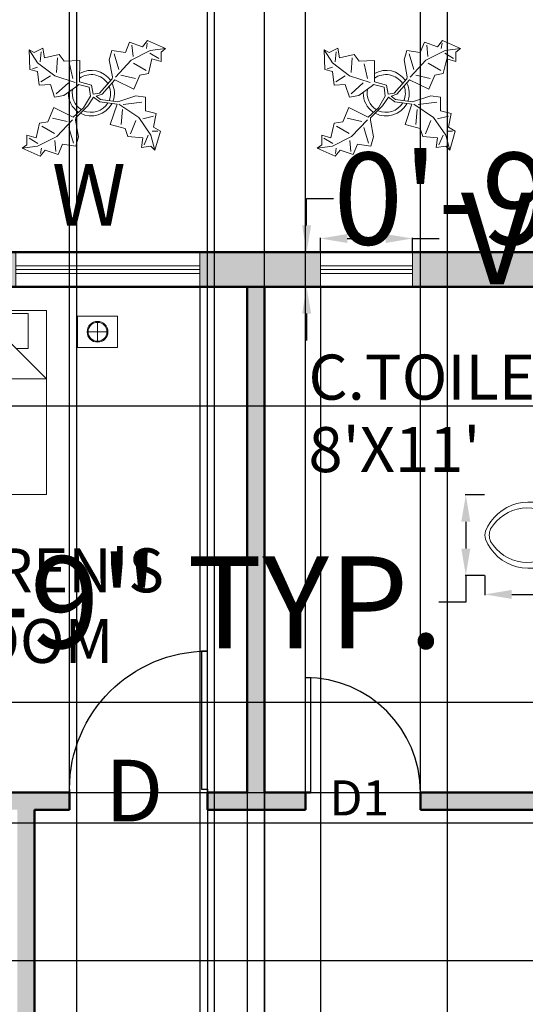
# Model space of a CAD drawing. Units: inches. Extents: x -166 to 1001, y 0 to 688.
# Tile 5 of 11: x 97 to 229, y 287 to 544. Entities that reach past the tile are written whole.
import ezdxf

# ---------------------------------------------------------------- set-up
doc = ezdxf.new("R2010")
doc.units = ezdxf.units.IN
doc.header["$MEASUREMENT"] = 0
for name, color, linetype, lineweight in [('A-ANNO-DIMS', 1, 'Continuous', 18), ('A-ANNO-TEXT', 2, 'Continuous', 25), ('A-AREA-IDEN', 2, 'Continuous', 25), ('A-DOOR', 6, 'Continuous', 25), ('A-FLOR-FIXT', 11, 'Continuous', 18), ('A-GLAZ', 130, 'Continuous', 18), ('A-GLAZ-VENT', 130, 'Continuous', 18), ('A-WALL-PATT', 5, 'Continuous', 13), ('FURNITURE', 11, 'Continuous', 18), ('TREES', 80, 'Continuous', 13), ('WALLS', 250, 'Continuous', 50)]:
    doc.layers.add(name, color=color, linetype=linetype, lineweight=lineweight)
doc.styles.get("Standard").update_dxf_attribs({"font": 'arial.ttf'})
doc.dimstyles.get("Standard").update_dxf_attribs({"dimtxt": 24, "dimasz": 7, "dimexe": 0.18, "dimexo": 0.0625, "dimgap": 0.09, "dimtad": 0, "dimtih": 1, "dimtoh": 1, "dimdec": 0, "dimzin": 0, "dimdsep": 46, "dimlunit": 3, "dimtxsty": 'Standard', "dimcen": 0.09, "dimadec": 0, "dimazin": 0, "dimtfac": 1, "dimtdec": 0, "dimtofl": 0, "dimtmove": 0, "dimatfit": 3, "dimfxl": 1, "dimtolj": 1, "dimtzin": 0, "dimarcsym": 0})

# ---------------------------------------------------------------- blocks, each defined once
blk = doc.blocks.new('*U6')
for p, q in [((0, 0), (0, -6)), ((40, 0), (40, -6))]:
    blk.add_line(p, q)
blk.add_lwpolyline([(0, 0), (0, 40), (1.75, 40), (1.75, 0)], close=True)
blk.add_arc((0, 0), 40, 0, 90)
blk = doc.blocks.new('Bed - Queen')
for p, q in [((0, -80.00003), (0, 0)), ((0, 0), (59.99999, 0)), ((59.99999, 0), (59.99999, -80.00003)), ((7.99999, -1.2), (28.79998, -1.2)), ((7.99999, -14.4), (7.99999, -1.2)), ((28.79998, -1.2), (28.79998, -14.4)), ((31.19999, -1.2), (51.99999, -1.2)), ((31.19999, -14.4), (31.19999, -1.2)), ((51.99999, -1.2), (51.99999, -16.4)), ((0, -14.4), (44.8, -14.4)), ((44.8, -16.8), (0, -16.8)), ((59.99999, -29.6), (44.8, -14.4)), ((44.8, -14.4), (44.8, -29.6)), ((51.99999, -16.4), (46.79936, -16.4)), ((44.8, -29.6), (59.99999, -29.6)), ((59.99999, -80.00003), (0, -80.00003))]:
    blk.add_line(p, q)
blk = doc.blocks.new('Toilet - top')
for p, q in [((9.5, -6), (9.5, -2)), ((-10, -8.5), (-8, -8.5)), ((-10, -9.5), (-10, -8.5)), ((-7, -9.5), (-10, -9.5)), ((-8, -8.5), (-8, -8)), ((-7, -8), (-7, -9.5)), ((-4, -8), (-6, -14)), ((4, -8), (6, -14)), ((4, -14), (-4, -14))]:
    blk.add_line(p, q)
blk.add_lwpolyline([(10.5, -8), (10.5, 0), (-10.5, 0), (-10.5, -8)], close=True)
for points in [[(-9.5, -2), (-9.5, -6)], [(8.5, -1), (-8.5, -1)], [(-8.5, -7), (8.5, -7)]]:
    blk.add_lwpolyline(points)
for centre, radius, start, end in [((-8.62, -1.88), 0.884, 81.8699, 188.1301), ((8.62, -1.88), 0.884, 351.8699, 98.1301), ((-8.62, -6.12), 0.884, 171.8699, 278.1301), ((8.62, -6.12), 0.884, 261.8699, 8.1301), ((3.52, -21.58), 12.17, 141.4691, 247.9714), ((4.2, -21.82), 11.33, 136.3677, 238.9468), ((-3.52, -21.58), 12.17, 292.0284, 38.5307), ((-4.2, -21.82), 11.33, 301.053, 43.6321), ((0, -27.88), 4, 245.7318, 294.2682), ((0, -29), 4, 254.8605, 285.1395)]:
    blk.add_arc(centre, radius, start, end)
blk = doc.blocks.new('Plant - Rubber or Philodendron')
for p, q in [((8.8871, 10.7908), (9.9809, 13.4933)), ((9.9809, 13.4933), (13.3837, 12.301)), ((13.3837, 12.301), (14.68, 13.9039)), ((14.5816, 13.2037), (14.3848, 11.8033)), ((14.68, 13.9039), (19.3848, 11.8146)), ((-16.2005, 11.4774), (-13.9899, 8.1064)), ((-16.2005, 11.4774), (-14.8639, 10.7964)), ((-16.0159, 6.3329), (-16.2005, 11.4774)), ((-14.8639, 10.7964), (-12.6195, 11.8975)), ((-13.3174, 8.325), (-13.0735, 11.0065)), ((-12.6195, 11.8975), (-12.1909, 9.4345)), ((-12.1909, 9.4345), (-8.3829, 10.3)), ((-8.3829, 10.3), (-7.0549, 8.501)), ((4.6914, 8.8812), (5.3859, 11.2828)), ((5.3859, 11.2828), (8.8871, 10.7908)), ((5.9878, 10.4842), (7.1971, 6.3869)), ((15.3859, 11.3055), (10.3916, 8.7942)), ((10.5828, 12.6946), (10.8893, 9.7953)), ((15.2875, 10.6053), (17.5907, 9.2105)), ((19.3848, 11.8146), (15.3859, 11.3055)), ((19.3848, 11.8146), (18.1868, 10.9119)), ((18.1868, 10.9119), (18.1925, 8.4119)), ((-13.9899, 8.1064), (-9.5434, 4.7185)), ((-8.8369, 9.409), (-9.0894, 5.6095)), ((-7.0549, 8.501), (-3.0284, 8.6941)), ((-4.8529, 4.012), (-5.7184, 7.82)), ((-3.0284, 8.6941), (-3.0709, 3.1041)), ((4.6914, 8.8812), (5.5014, 4.4831)), ((10.3916, 8.7942), (6.2847, 4.4028)), ((14.2977, 6.1031), (10.9934, 7.9956)), ((15.7909, 9.1065), (14.8995, 5.3044)), ((18.1925, 8.4119), (15.7909, 9.1065)), ((-14.0069, 5.8704), (-16.0159, 6.3329)), ((-15.3434, 6.5514), (-13.9984, 6.9884)), ((-13.5868, 2.2894), (-14.0069, 5.8704)), ((14.8995, 5.3044), (12.7005, 4.8994)), ((-13.1329, 3.1804), (-10.6614, 4.727)), ((-9.5434, 4.7185), (-4.1917, 2.9888)), ((-9.1318, 0.0195), (-5.9793, 2.9025)), ((-3.0709, 3.1041), (0.0797, 2.3163)), ((2.1141, 0.2298), (5.4346, 3.9146)), ((6.1032, 3.6844), (2.8262, -0.031)), ((5.4346, 3.9146), (5.5014, 4.4831)), ((11.1089, 1.1958), (6.1032, 3.6844)), ((7.7005, 4.8881), (11.5025, 3.9967)), ((12.7005, 4.8994), (11.1089, 1.1958)), ((-10.6784, 2.491), (-13.5868, 2.2894)), ((-9.5858, -0.8715), (-10.6784, 2.491)), ((-7.1228, -0.443), (-3.5248, 2.2131)), ((-3.5248, 2.2131), (-3.3011, 2.4355)), ((-3.3011, 2.4355), (-0.5306, 1.7947)), ((-0.5306, 1.7947), (-0.2255, -0.5527)), ((-0.5306, 1.7947), (-0.5306, 1.7947)), ((0.0797, 2.3163), (0.4866, -0.031)), ((0.4866, -0.031), (2.1141, 0.2298)), ((-7.1228, -0.443), (-9.5858, -0.8715)), ((-2.019, -3.6148), (-0.2255, -0.5527)), ((-0.9375, -3.1608), (0.5883, -0.8135)), ((0.5883, -0.8135), (2.2447, -2.0916)), ((2.8262, -0.031), (1.3003, -0.5527)), ((1.3003, -0.5527), (2.4193, -1.4655)), ((2.2447, -2.0916), (6.7108, -2.6626)), ((2.4193, -1.4655), (6.895, -2.1175)), ((11.6605, -0.5413), (6.895, -2.1175)), ((8.3544, -2.7453), (13.1973, -2.1704)), ((11.6605, -0.5413), (14.1354, -0.8948)), ((14.1354, -0.8948), (14.1354, -4.4304)), ((-11.3237, -7.2629), (-9.7321, -3.5593)), ((-9.7321, -3.5593), (-4.7264, -6.0479)), ((-2.019, -3.6148), (-4.7264, -6.0479)), ((-4.0579, -6.2781), (-0.9375, -3.1608)), ((4.943, -7.9659), (6.7108, -2.6626)), ((12.3677, -6.1981), (7.219, -2.6772)), ((8.125, -4.0768), (7.7715, -7.9659)), ((14.1354, -4.4304), (16.9638, -5.1375)), ((16.9638, -5.1375), (16.2567, -8.673)), ((-14.4141, -11.4699), (-13.5228, -7.6679)), ((-13.5228, -7.6679), (-11.3237, -7.2629)), ((-6.3237, -7.2516), (-10.1257, -6.3602)), ((-9.0148, -11.1577), (-4.9047, -6.8122)), ((-4.1246, -6.8466), (-4.0579, -6.2781)), ((-3.3146, -11.2447), (-4.1246, -6.8466)), ((10.2463, -10.4408), (11.6605, -6.9053)), ((15.5496, -10.7943), (12.3677, -6.1981)), ((16.2567, -5.8446), (13.4283, -6.5517)), ((-12.921, -8.4665), (-9.6166, -10.359)), ((-4.611, -12.8477), (-5.8203, -8.7504)), ((8.8321, -9.0266), (4.943, -7.9659)), ((9.5392, -11.1479), (8.8321, -9.0266)), ((17.3174, -9.7337), (15.9032, -9.7337)), ((16.2567, -8.673), (18.0245, -9.7337)), ((18.0245, -9.7337), (16.6103, -14.6834)), ((-16.8157, -10.7754), (-14.4141, -11.4699)), ((-16.8101, -13.2754), (-16.8157, -10.7754)), ((-13.9107, -12.9688), (-16.2139, -11.574)), ((-14.0091, -13.669), (-9.0148, -11.1577)), ((-9.206, -15.0581), (-9.5126, -12.1588)), ((-3.3146, -11.2447), (-4.0092, -13.6463)), ((13.4283, -11.5015), (9.5392, -11.1479)), ((13.0748, -13.9763), (13.4283, -11.5015)), ((14.8425, -10.7943), (13.7819, -13.2692)), ((16.6103, -14.6834), (15.5496, -10.7943)), ((-18.008, -14.1781), (-16.8101, -13.2754)), ((-18.008, -14.1781), (-14.0091, -13.669)), ((-13.3032, -16.2674), (-18.008, -14.1781)), ((-12.0069, -14.6645), (-13.3032, -16.2674)), ((-13.2048, -15.5672), (-13.008, -14.1668)), ((-8.6042, -15.8568), (-12.0069, -14.6645)), ((-7.5103, -13.1543), (-8.6042, -15.8568)), ((-4.0092, -13.6463), (-7.5103, -13.1543)), ((15.5496, -13.6228), (13.0748, -13.9763)), ((16.6103, -14.6834), (15.5496, -13.6228))]:
    blk.add_line(p, q)
for centre, radius, start, end in [((0, 0), 6.1275, 34.37569, 120.1028), ((-0.0601, -0.2075), 5.2461, 33.82192, 124.9414), ((-0.098, 0.1364), 6.1288, 341.2017, 26.09184), ((0.0308, 0.1664), 6, 178.6147, 235.1169), ((0.0308, 0.1664), 5, 168.1647, 238.6725), ((-0.2664, 0.1682), 5.2775, 338.4094, 20.03007), ((-0.1102, 0.4886), 5.2883, 247.3711, 327.472), ((-0.0234, 0.3825), 6.1492, 242.5812, 331.2714)]:
    blk.add_arc(centre, radius, start, end)
blk = doc.blocks.new('WIN-48IN')
for p, q in [((0, 4.5), (0, 9)), ((0, 9), (0, 0)), ((48, 9), (48, 0)), ((0, 5.5), (48, 5.5)), ((0, 4.5), (48, 4.5)), ((0, 3.5), (48, 3.5))]:
    blk.add_line(p, q)
blk = doc.blocks.new('VENT-24IN')
for p, q in [((0, 4.5), (0, 9)), ((0, 9), (0, 0)), ((24, 9), (24, 0)), ((0, 5.5), (24, 5.5)), ((0, 4.5), (24, 4.5)), ((0, 3.5), (24, 3.5))]:
    blk.add_line(p, q)
blk = doc.blocks.new('BEDSIDE-TABLE-LAMP')
for p, q in [((5.2, 1.64), (5.2, 6.55)), ((2.75, 4.1), (7.66, 4.1))]:
    blk.add_line(p, q)
blk.add_lwpolyline([(0, 8.19), (10.4, 8.19), (10.4, 0), (0, 0)], close=True)
for radius in [2.71, 2.71, 2.71, 2.46]:
    blk.add_circle((5.2, 4.1), radius)
blk = doc.blocks.new('*D19')
at = {"layer": 'A-ANNO-DIMS', "color": 0, "lineweight": -2, "transparency": 16777216}
for p, q in [((175.47, 483.8), (175.47, 487.52)), ((182.47, 487.34), (192.47, 487.34)), ((199.47, 483.8), (199.47, 487.52)), ((199.47, 487.34), (206.47, 487.34))]:
    blk.add_line(p, q, dxfattribs=at)
at = {"layer": 'A-ANNO-DIMS', "color": 0, "transparency": 16777216}
for points in [[(182.47, 488.51), (182.47, 486.17), (175.47, 487.34)], [(192.47, 488.51), (192.47, 486.17), (199.47, 487.34)]]:
    blk.add_solid(points, dxfattribs=at)
at = {"layer": 'Defpoints', "color": 0, "transparency": 16777216}
for p in [(199.47, 487.34), (175.47, 483.74), (199.47, 483.74)]:
    blk.add_point(p, dxfattribs=at)
at = {"layer": 'A-ANNO-DIMS', "color": 0, "transparency": 16777216, "insert": (329.7, 487.34), "char_height": 24, "attachment_point": 5}
blk.add_mtext('\\A1;VENT 2\'-0" TYP.', dxfattribs=at)
blk = doc.blocks.new('*D20')
at = {"layer": 'A-ANNO-DIMS', "color": 0, "lineweight": -2, "transparency": 16777216}
for p, q in [((171.87, 490.74), (171.87, 497.74)), ((171.87, 497.74), (178.87, 497.74)), ((175.41, 483.74), (171.69, 483.74)), ((175.41, 474.74), (171.69, 474.74)), ((171.87, 467.74), (171.87, 460.74))]:
    blk.add_line(p, q, dxfattribs=at)
at = {"layer": 'A-ANNO-DIMS', "color": 0, "transparency": 16777216}
for points in [[(170.71, 490.74), (173.04, 490.74), (171.87, 483.74)], [(170.71, 467.74), (173.04, 467.74), (171.87, 474.74)]]:
    blk.add_solid(points, dxfattribs=at)
at = {"layer": 'Defpoints', "color": 0, "transparency": 16777216}
for p in [(171.87, 483.74), (175.47, 483.74), (175.47, 474.74)]:
    blk.add_point(p, dxfattribs=at)
at = {"layer": 'A-ANNO-DIMS', "color": 0, "transparency": 16777216, "insert": (252.11, 497.74), "char_height": 24, "attachment_point": 5}
blk.add_mtext('\\A1;0\'-9" TYP.', dxfattribs=at)
blk = doc.blocks.new('*D25')
at = {"layer": 'A-ANNO-DIMS', "color": 0, "lineweight": -2, "transparency": 16777216}
for p, q in [((218.36, 399.34), (218.36, 394.26)), ((251.4, 399.34), (251.4, 394.26)), ((225.36, 394.44), (244.4, 394.44)), ((251.4, 394.44), (258.4, 394.44))]:
    blk.add_line(p, q, dxfattribs=at)
at = {"layer": 'A-ANNO-DIMS', "color": 0, "transparency": 16777216}
for points in [[(225.36, 395.61), (225.36, 393.27), (218.36, 394.44)], [(244.4, 395.61), (244.4, 393.27), (251.4, 394.44)]]:
    blk.add_solid(points, dxfattribs=at)
at = {"layer": 'Defpoints', "color": 0, "transparency": 16777216}
for p in [(218.36, 399.4), (251.4, 399.4), (251.4, 394.44)]:
    blk.add_point(p, dxfattribs=at)
at = {"layer": 'A-ANNO-DIMS', "color": 0, "transparency": 16777216, "insert": (364.72, 394.44), "char_height": 24, "attachment_point": 5}
blk.add_mtext('\\A1;WC 2\'-9" TYP.', dxfattribs=at)
blk = doc.blocks.new('*D26')
at = {"layer": 'A-ANNO-DIMS', "color": 0, "lineweight": -2, "transparency": 16777216}
for p, q in [((218.29, 420.4), (213.22, 420.4)), ((213.4, 413.4), (213.4, 406.4)), ((218.29, 399.4), (213.22, 399.4)), ((213.4, 399.4), (213.4, 392.4)), ((213.4, 392.4), (206.4, 392.4))]:
    blk.add_line(p, q, dxfattribs=at)
at = {"layer": 'A-ANNO-DIMS', "color": 0, "transparency": 16777216}
for points in [[(212.23, 413.4), (214.57, 413.4), (213.4, 420.4)], [(212.23, 406.4), (214.57, 406.4), (213.4, 399.4)]]:
    blk.add_solid(points, dxfattribs=at)
at = {"layer": 'Defpoints', "color": 0, "transparency": 16777216}
for p in [(218.36, 420.4), (213.4, 399.4), (218.36, 399.4)]:
    blk.add_point(p, dxfattribs=at)
at = {"layer": 'A-ANNO-DIMS', "color": 0, "transparency": 16777216, "insert": (134.29, 392.4), "char_height": 24, "attachment_point": 5}
blk.add_mtext('\\A1;1\'-9" TYP.', dxfattribs=at)
blk = doc.blocks.new('*D35')
at = {"layer": 'A-ANNO-DIMS', "color": 0, "lineweight": -2, "transparency": 16777216}
for p, q in [((15.38, 483.8), (15.38, 593.07)), ((22.38, 592.89), (207.38, 592.89)), ((531.88, 592.89), (346.89, 592.89)), ((538.88, 483.8), (538.88, 593.07))]:
    blk.add_line(p, q, dxfattribs=at)
at = {"layer": 'A-ANNO-DIMS', "color": 0, "transparency": 16777216}
for points in [[(22.38, 594.06), (22.38, 591.72), (15.38, 592.89)], [(531.88, 594.06), (531.88, 591.72), (538.88, 592.89)]]:
    blk.add_solid(points, dxfattribs=at)
at = {"layer": 'Defpoints', "color": 0, "transparency": 16777216}
for p in [(538.88, 592.89), (15.38, 483.74), (538.88, 483.74)]:
    blk.add_point(p, dxfattribs=at)
at = {"layer": 'A-ANNO-DIMS', "color": 0, "transparency": 16777216, "insert": (277.13, 592.89), "char_height": 24, "attachment_point": 5}
blk.add_mtext('\\A1;43\'-7 1/2"', dxfattribs=at)
blk = doc.blocks.new('*D43')
at = {"layer": 'A-ANNO-DIMS', "color": 0, "lineweight": -2, "transparency": 16777216}
for p, q in [((160.88, 257.49), (160.88, 593.07)), ((167.88, 592.89), (201.62, 592.89)), ((208.62, 257.49), (208.62, 593.07)), ((208.62, 592.89), (215.62, 592.89))]:
    blk.add_line(p, q, dxfattribs=at)
at = {"layer": 'A-ANNO-DIMS', "color": 0, "transparency": 16777216}
for points in [[(167.88, 594.06), (167.88, 591.72), (160.88, 592.89)], [(201.62, 594.06), (201.62, 591.72), (208.62, 592.89)]]:
    blk.add_solid(points, dxfattribs=at)
at = {"layer": 'Defpoints', "color": 0, "transparency": 16777216}
for p in [(208.62, 592.89), (160.88, 257.42), (208.62, 257.42)]:
    blk.add_point(p, dxfattribs=at)
at = {"layer": 'A-ANNO-DIMS', "color": 0, "transparency": 16777216, "insert": (284.89, 592.89), "char_height": 24, "attachment_point": 5}
blk.add_mtext('\\A1;3\'-11 1/2"', dxfattribs=at)
blk = doc.blocks.new('*D44')
at = {"layer": 'A-ANNO-DIMS', "color": 0, "lineweight": -2, "transparency": 16777216}
for p, q in [((144.05, 474.68), (144.05, 35.41)), ((156.38, 474.68), (156.38, 35.41)), ((137.05, 35.59), (130.05, 35.59)), ((163.38, 35.59), (170.38, 35.59))]:
    blk.add_line(p, q, dxfattribs=at)
at = {"layer": 'A-ANNO-DIMS', "color": 0, "transparency": 16777216}
for points in [[(137.05, 36.76), (137.05, 34.42), (144.05, 35.59)], [(163.38, 36.76), (163.38, 34.42), (156.38, 35.59)]]:
    blk.add_solid(points, dxfattribs=at)
at = {"layer": 'Defpoints', "color": 0, "transparency": 16777216}
for p in [(144.05, 474.74), (156.38, 474.74), (156.38, 35.59)]:
    blk.add_point(p, dxfattribs=at)
at = {"layer": 'A-ANNO-DIMS', "color": 0, "transparency": 16777216, "insert": (229.2, 35.59), "char_height": 24, "attachment_point": 5}
blk.add_mtext('\\A1;1\'-0 1/2"', dxfattribs=at)
blk = doc.blocks.new('*D45')
at = {"layer": 'A-ANNO-DIMS', "color": 0, "lineweight": -2, "transparency": 16777216}
for p, q in [((160.88, 474.68), (160.88, 35.41)), ((175.47, 474.68), (175.47, 35.41)), ((167.88, 35.59), (168.47, 35.59)), ((175.47, 35.59), (182.47, 35.59))]:
    blk.add_line(p, q, dxfattribs=at)
at = {"layer": 'A-ANNO-DIMS', "color": 0, "transparency": 16777216}
for points in [[(167.88, 36.76), (167.88, 34.42), (160.88, 35.59)], [(168.47, 36.76), (168.47, 34.42), (175.47, 35.59)]]:
    blk.add_solid(points, dxfattribs=at)
at = {"layer": 'Defpoints', "color": 0, "transparency": 16777216}
for p in [(160.88, 474.74), (175.47, 474.74), (175.47, 35.59)]:
    blk.add_point(p, dxfattribs=at)
at = {"layer": 'A-ANNO-DIMS', "color": 0, "transparency": 16777216, "insert": (241.29, 35.59), "char_height": 24, "attachment_point": 5}
blk.add_mtext('\\A1;1\'-2 1/2"', dxfattribs=at)
blk = doc.blocks.new('*D52')
at = {"layer": 'A-ANNO-DIMS', "color": 0, "lineweight": -2, "transparency": 16777216}
for p, q in [((675.03, 366.29), (675.03, 373.29)), ((675.03, 373.29), (682.03, 373.29)), ((24.44, 366.29), (675.21, 366.29)), ((675.03, 349.74), (675.03, 359.29)), ((24.44, 342.74), (675.21, 342.74))]:
    blk.add_line(p, q, dxfattribs=at)
at = {"layer": 'A-ANNO-DIMS', "color": 0, "transparency": 16777216}
for points in [[(673.87, 359.29), (676.2, 359.29), (675.03, 366.29)], [(673.87, 349.74), (676.2, 349.74), (675.03, 342.74)]]:
    blk.add_solid(points, dxfattribs=at)
at = {"layer": 'Defpoints', "color": 0, "transparency": 16777216}
for p in [(24.38, 366.29), (675.03, 366.29), (24.38, 342.74)]:
    blk.add_point(p, dxfattribs=at)
at = {"layer": 'A-ANNO-DIMS', "color": 0, "transparency": 16777216, "insert": (750.18, 373.29), "char_height": 24, "attachment_point": 5}
blk.add_mtext('\\A1;1\'-11 1/2"', dxfattribs=at)
blk = doc.blocks.new('*D55')
at = {"layer": 'A-ANNO-DIMS', "color": 0, "lineweight": -2, "transparency": 16777216}
for p, q in [((-120.77, 341.73), (-120.77, 348.73)), ((529.82, 334.73), (-120.95, 334.73)), ((529.82, 298.79), (-120.95, 298.79)), ((-120.77, 291.79), (-120.77, 284.79))]:
    blk.add_line(p, q, dxfattribs=at)
at = {"layer": 'A-ANNO-DIMS', "color": 0, "transparency": 16777216}
for points in [[(-121.93, 341.73), (-119.6, 341.73), (-120.77, 334.73)], [(-121.93, 291.79), (-119.6, 291.79), (-120.77, 298.79)]]:
    blk.add_solid(points, dxfattribs=at)
at = {"layer": 'Defpoints', "color": 0, "transparency": 16777216}
for p in [(-120.77, 334.73), (529.88, 334.73), (529.88, 298.79)]:
    blk.add_point(p, dxfattribs=at)
at = {"layer": 'A-ANNO-DIMS', "color": 0, "transparency": 16777216, "insert": (-120.77, 316.76), "char_height": 24, "attachment_point": 5}
blk.add_mtext('\\A1;3\'-0"', dxfattribs=at)
blk = doc.blocks.new('*D59')
at = {"layer": 'A-ANNO-DIMS', "color": 0, "lineweight": -2, "transparency": 16777216}
for p, q in [((110.03, 342.8), (110.03, 593.07)), ((117.03, 592.89), (139.03, 592.89)), ((146.03, 342.8), (146.03, 593.07)), ((146.03, 592.89), (153.03, 592.89))]:
    blk.add_line(p, q, dxfattribs=at)
at = {"layer": 'A-ANNO-DIMS', "color": 0, "transparency": 16777216}
for points in [[(117.03, 594.06), (117.03, 591.72), (110.03, 592.89)], [(139.03, 594.06), (139.03, 591.72), (146.03, 592.89)]]:
    blk.add_solid(points, dxfattribs=at)
at = {"layer": 'Defpoints', "color": 0, "transparency": 16777216}
for p in [(146.03, 592.89), (110.03, 342.74), (146.03, 342.74)]:
    blk.add_point(p, dxfattribs=at)
at = {"layer": 'A-ANNO-DIMS', "color": 0, "transparency": 16777216, "insert": (185.01, 592.89), "char_height": 24, "attachment_point": 5}
blk.add_mtext('\\A1;3\'-0"', dxfattribs=at)
blk = doc.blocks.new('*D60')
at = {"layer": 'A-ANNO-DIMS', "color": 0, "lineweight": -2, "transparency": 16777216}
for p, q in [((156.38, 342.68), (156.38, 35.41)), ((146.03, 338.18), (146.03, 35.41)), ((139.03, 35.59), (132.03, 35.59)), ((163.38, 35.59), (170.38, 35.59))]:
    blk.add_line(p, q, dxfattribs=at)
at = {"layer": 'A-ANNO-DIMS', "color": 0, "transparency": 16777216}
for points in [[(139.03, 36.76), (139.03, 34.42), (146.03, 35.59)], [(163.38, 36.76), (163.38, 34.42), (156.38, 35.59)]]:
    blk.add_solid(points, dxfattribs=at)
at = {"layer": 'Defpoints', "color": 0, "transparency": 16777216}
for p in [(156.38, 342.74), (146.03, 338.24), (156.38, 35.59)]:
    blk.add_point(p, dxfattribs=at)
at = {"layer": 'A-ANNO-DIMS', "color": 0, "transparency": 16777216, "insert": (239.66, 35.59), "char_height": 24, "attachment_point": 5}
blk.add_mtext('\\A1;0\'-10 1/2"', dxfattribs=at)
blk = doc.blocks.new('*D61')
at = {"layer": 'A-ANNO-DIMS', "color": 0, "lineweight": -2, "transparency": 16777216}
for p, q in [((171.55, 342.8), (171.55, 593.07)), ((178.55, 592.89), (194.55, 592.89)), ((201.55, 342.8), (201.55, 593.07)), ((201.55, 592.89), (208.55, 592.89))]:
    blk.add_line(p, q, dxfattribs=at)
at = {"layer": 'A-ANNO-DIMS', "color": 0, "transparency": 16777216}
for points in [[(178.55, 594.06), (178.55, 591.72), (171.55, 592.89)], [(194.55, 594.06), (194.55, 591.72), (201.55, 592.89)]]:
    blk.add_solid(points, dxfattribs=at)
at = {"layer": 'Defpoints', "color": 0, "transparency": 16777216}
for p in [(201.55, 592.89), (171.55, 342.74), (201.55, 342.74)]:
    blk.add_point(p, dxfattribs=at)
at = {"layer": 'A-ANNO-DIMS', "color": 0, "transparency": 16777216, "insert": (240.75, 592.89), "char_height": 24, "attachment_point": 5}
blk.add_mtext('\\A1;2\'-6"', dxfattribs=at)
blk = doc.blocks.new('*D62')
at = {"layer": 'A-ANNO-DIMS', "color": 0, "lineweight": -2, "transparency": 16777216}
for p, q in [((201.55, 342.8), (201.55, 593.07)), ((208.55, 592.89), (249.88, 592.89)), ((256.88, 342.8), (256.88, 593.07)), ((256.88, 592.89), (263.88, 592.89))]:
    blk.add_line(p, q, dxfattribs=at)
at = {"layer": 'A-ANNO-DIMS', "color": 0, "transparency": 16777216}
for points in [[(208.55, 594.06), (208.55, 591.72), (201.55, 592.89)], [(249.88, 594.06), (249.88, 591.72), (256.88, 592.89)]]:
    blk.add_solid(points, dxfattribs=at)
at = {"layer": 'Defpoints', "color": 0, "transparency": 16777216}
for p in [(256.88, 592.89), (201.55, 342.74), (256.88, 342.74)]:
    blk.add_point(p, dxfattribs=at)
at = {"layer": 'A-ANNO-DIMS', "color": 0, "transparency": 16777216, "insert": (324.32, 592.89), "char_height": 24, "attachment_point": 5}
blk.add_mtext('\\A1;4\'-7 1/2"', dxfattribs=at)
blk = doc.blocks.new('*D67')
at = {"layer": 'A-ANNO-DIMS', "color": 0, "lineweight": -2, "transparency": 16777216}
for p, q in [((44.93, 278.3), (44.93, 593.07)), ((51.93, 592.89), (67.93, 592.89)), ((74.93, 278.3), (74.93, 593.07)), ((74.93, 592.89), (81.93, 592.89))]:
    blk.add_line(p, q, dxfattribs=at)
at = {"layer": 'A-ANNO-DIMS', "color": 0, "transparency": 16777216}
for points in [[(51.93, 594.06), (51.93, 591.72), (44.93, 592.89)], [(67.93, 594.06), (67.93, 591.72), (74.93, 592.89)]]:
    blk.add_solid(points, dxfattribs=at)
at = {"layer": 'Defpoints', "color": 0, "transparency": 16777216}
for p in [(74.93, 592.89), (44.93, 278.24), (74.93, 278.24)]:
    blk.add_point(p, dxfattribs=at)
at = {"layer": 'A-ANNO-DIMS', "color": 0, "transparency": 16777216, "insert": (114.12, 592.89), "char_height": 24, "attachment_point": 5}
blk.add_mtext('\\A1;2\'-6"', dxfattribs=at)
blk = doc.blocks.new('*D69')
at = {"layer": 'A-ANNO-DIMS', "color": 0, "lineweight": -2, "transparency": 16777216}
for p, q in [((111.92, 278.3), (111.92, 593.07)), ((118.92, 592.89), (140.87, 592.89)), ((147.87, 278.3), (147.87, 593.07)), ((147.87, 592.89), (154.87, 592.89))]:
    blk.add_line(p, q, dxfattribs=at)
at = {"layer": 'A-ANNO-DIMS', "color": 0, "transparency": 16777216}
for points in [[(118.92, 594.06), (118.92, 591.72), (111.92, 592.89)], [(140.87, 594.06), (140.87, 591.72), (147.87, 592.89)]]:
    blk.add_solid(points, dxfattribs=at)
at = {"layer": 'Defpoints', "color": 0, "transparency": 16777216}
for p in [(147.87, 592.89), (111.92, 278.24), (147.87, 278.24)]:
    blk.add_point(p, dxfattribs=at)
at = {"layer": 'A-ANNO-DIMS', "color": 0, "transparency": 16777216, "insert": (186.85, 592.89), "char_height": 24, "attachment_point": 5}
blk.add_mtext('\\A1;3\'-0"', dxfattribs=at)
blk = doc.blocks.new('*D75')
at = {"layer": 'A-ANNO-DIMS', "color": 0, "lineweight": -2, "transparency": 16777216}
for p, q in [((-120.77, 481.74), (-120.77, 488.74)), ((529.82, 474.74), (-120.95, 474.74)), ((529.82, 443.59), (-120.95, 443.59)), ((-120.77, 436.59), (-120.77, 429.59))]:
    blk.add_line(p, q, dxfattribs=at)
at = {"layer": 'A-ANNO-DIMS', "color": 0, "transparency": 16777216}
for points in [[(-121.93, 481.74), (-119.6, 481.74), (-120.77, 474.74)], [(-121.93, 436.59), (-119.6, 436.59), (-120.77, 443.59)]]:
    blk.add_solid(points, dxfattribs=at)
at = {"layer": 'Defpoints', "color": 0, "transparency": 16777216}
for p in [(529.88, 474.74), (-120.77, 443.59), (529.88, 443.59)]:
    blk.add_point(p, dxfattribs=at)
at = {"layer": 'A-ANNO-DIMS', "color": 0, "transparency": 16777216, "insert": (-120.77, 459.16), "char_height": 24, "attachment_point": 5}
blk.add_mtext('\\A1;2\'-7"', dxfattribs=at)
blk = doc.blocks.new('*D78')
at = {"layer": 'A-ANNO-DIMS', "color": 0, "lineweight": -2, "transparency": 16777216}
for p, q in [((160.88, 153.8), (160.88, 593.07)), ((167.88, 592.89), (186.64, 592.89)), ((285.77, 592.89), (267.01, 592.89)), ((292.77, 153.8), (292.77, 593.07))]:
    blk.add_line(p, q, dxfattribs=at)
at = {"layer": 'A-ANNO-DIMS', "color": 0, "transparency": 16777216}
for points in [[(167.88, 594.06), (167.88, 591.72), (160.88, 592.89)], [(285.77, 594.06), (285.77, 591.72), (292.77, 592.89)]]:
    blk.add_solid(points, dxfattribs=at)
at = {"layer": 'Defpoints', "color": 0, "transparency": 16777216}
for p in [(292.77, 592.89), (160.88, 153.74), (292.77, 153.74)]:
    blk.add_point(p, dxfattribs=at)
at = {"layer": 'A-ANNO-DIMS', "color": 0, "transparency": 16777216, "insert": (226.83, 592.89), "char_height": 24, "attachment_point": 5}
blk.add_mtext('\\A1;11\'-0"', dxfattribs=at)

msp = doc.modelspace()

# ---------------------------------------------------------------- hatches: boundary and pattern name
at = {"layer": 'A-WALL-PATT'}
h = msp.add_hatch(color=256, dxfattribs=at)
h.dxf.hatch_style = 1
h.paths.add_polyline_path([(96.05, 483.74), (15.38, 483.74), (15.38, 414.29), (24.38, 414.29), (24.38, 474.74), (96.05, 474.74)])
h.paths.add_polyline_path([(175.47, 483.74), (144.05, 483.74), (144.05, 474.74), (156.38, 474.74), (175.47, 474.74)])
h.paths.add_polyline_path([(298.66, 483.74), (199.47, 483.74), (199.47, 474.74), (256.88, 474.74), (298.66, 474.74)])
h.paths.add_polyline_path([(430.46, 483.74), (346.66, 483.74), (346.66, 474.74), (393.38, 474.74), (430.46, 474.74)])
h.paths.add_polyline_path([(261.38, 474.74), (256.88, 474.74), (256.88, 342.74), (201.55, 342.74), (201.55, 338.24), (274.49, 338.24), (274.49, 342.74), (261.38, 342.74)])
h.paths.add_polyline_path([(160.88, 474.74), (156.38, 474.74), (156.38, 342.74), (146.03, 342.74), (146.03, 338.24), (171.55, 338.24), (171.55, 342.74), (160.88, 342.74)])
h.paths.add_polyline_path([(397.88, 474.74), (393.38, 474.74), (393.38, 383.21), (397.88, 383.21)])
h.paths.add_polyline_path([(538.88, 362.18), (529.88, 362.18), (529.88, 342.74), (397.88, 342.74), (397.88, 348.69), (393.38, 348.69), (393.38, 342.74), (384.24, 342.74), (384.24, 338.24), (529.88, 338.24), (529.88, 334.73), (538.88, 334.73)])
h.paths.add_polyline_path([(538.88, 483.74), (478.46, 483.74), (478.46, 474.74), (529.88, 474.74), (529.88, 410.18), (538.88, 410.18)])
h.paths.add_polyline_path([(538.88, 298.79), (529.88, 298.79), (529.88, 278.24), (442.61, 278.24), (442.61, 273.74), (529.88, 273.74), (529.88, 221.94), (538.88, 221.94)])
h.paths.add_polyline_path([(538.88, 173.94), (529.88, 173.94), (529.88, 153.74), (393.38, 153.74), (382.23, 153.74), (382.23, 144.74), (538.88, 144.74)])
h.paths.add_polyline_path([(397.88, 164.32), (393.38, 164.32), (393.38, 153.74), (397.88, 153.74)], flags=17)
h.paths.add_polyline_path([(397.88, 273.74), (406.66, 273.74), (406.66, 278.24), (393.38, 278.24), (393.38, 273.74), (393.38, 230.24), (316.88, 230.24), (316.88, 153.74), (321.38, 153.74), (321.38, 225.74), (393.38, 225.74), (393.38, 194.32), (397.88, 194.32)])
h.paths.add_polyline_path([(358.23, 153.74), (316.88, 153.74), (284.58, 153.74), (284.58, 144.74), (358.23, 144.74)])
h.paths.add_polyline_path([(224.58, 153.74), (156.38, 153.74), (149.31, 153.74), (149.31, 144.74), (224.58, 144.74)])
h.paths.add_polyline_path([(101.31, 153.74), (24.38, 153.74), (24.38, 168.41), (15.38, 168.41), (15.38, 144.74), (101.31, 144.74)])
h.paths.add_polyline_path([(160.88, 273.74), (160.88, 278.24), (147.87, 278.24), (147.87, 273.74), (156.38, 273.74), (156.38, 153.74), (160.88, 153.74)])
h.paths.add_polyline_path([(111.92, 278.24), (100.88, 278.24), (100.88, 338.24), (110.03, 338.24), (110.03, 342.74), (24.38, 342.74), (24.38, 366.29), (15.38, 366.29), (15.38, 216.41), (24.38, 216.41), (24.38, 273.74), (44.93, 273.74), (44.93, 278.24), (24.38, 278.24), (24.38, 338.24), (96.38, 338.24), (96.38, 278.24), (74.93, 278.24), (74.93, 273.74), (111.92, 273.74)])

# ---------------------------------------------------------------- linework, layer by layer
at = {"layer": 'WALLS'}
for p, q in [((15.38, 483.74), (538.88, 483.74)), ((24.38, 474.74), (156.38, 474.74)), ((156.38, 342.74), (156.38, 474.74)), ((156.38, 474.74), (256.88, 474.74)), ((160.88, 342.74), (160.88, 474.74)), ((24.38, 342.74), (110.03, 342.74)), ((110.03, 342.74), (110.03, 338.24)), ((146.03, 342.74), (156.38, 342.74)), ((146.03, 342.74), (146.03, 338.24)), ((160.88, 342.74), (172.86, 342.74)), ((171.55, 342.74), (171.55, 338.24)), ((201.55, 342.74), (256.88, 342.74)), ((201.55, 338.24), (201.55, 342.74)), ((100.88, 278.24), (100.88, 338.24)), ((100.88, 338.24), (110.03, 338.24)), ((146.03, 338.24), (171.55, 338.24)), ((201.55, 338.24), (529.88, 338.24))]:
    msp.add_line(p, q, dxfattribs=at)

# ---------------------------------------------------------------- block references
at = {"layer": 'A-DOOR'}
for p, xscale, yscale, zscale in [((146.03, 343.64), -0.8999999999999998, 0.8999999999999998, 0.8999999999999998), ((171.55, 342.74), 0.7500000000000006, 0.7500000000000006, 0.7500000000000006)]:
    msp.add_blockref('*U6', p, dxfattribs=dict(at, xscale=xscale, yscale=yscale, zscale=zscale))
at = {"layer": 'A-FLOR-FIXT', "rotation": 270}
msp.add_blockref('Toilet - top', (251.4, 409.9), dxfattribs=at)
at = {"layer": 'A-GLAZ'}
msp.add_blockref('WIN-48IN', (96.05, 474.74), dxfattribs=at)
at = {"layer": 'A-GLAZ-VENT'}
msp.add_blockref('VENT-24IN', (175.47, 474.74), dxfattribs=at)
at = {"layer": 'FURNITURE', "xscale": 0.6000001000000168, "yscale": 0.6000001000000168, "zscale": 0.6000001000000168}
msp.add_blockref('Bed - Queen', (68.02, 468.51), dxfattribs=at)
at = {"layer": 'FURNITURE'}
msp.add_blockref('BEDSIDE-TABLE-LAMP', (112.14, 458.89), dxfattribs=at)
at = {"layer": 'TREES'}
for p in [(115.71, 525.09), (192.62, 525.09)]:
    msp.add_blockref('Plant - Rubber or Philodendron', p, dxfattribs=at)

# ---------------------------------------------------------------- texts
at = {"layer": 'A-ANNO-TEXT'}
for s, height, p in [('W ', 16.096, (105.44, 490.68)), ('D', 16.1, (119.36, 335.18)), ('D1', 9.17, (177.86, 336.74))]:
    msp.add_text(s, height=height, dxfattribs=at).set_placement(p)
at = {"layer": 'A-AREA-IDEN'}
for s, height, p in [('C.TOILET', 11.769, (172.36, 445.27)), ("8'X11'", 11.769, (172.36, 426.36)), ("CHILDREN'S", 11.478, (45.26, 394.98)), ('BEDROOM', 11.478, (45.26, 376.54))]:
    msp.add_text(s, height=height, dxfattribs=at).set_placement(p)

# ---------------------------------------------------------------- dimensions: what is measured, and where the dimension line sits
at = {"layer": 'A-ANNO-DIMS'}
for base, p1, p2, picture, middle in [((538.88, 592.89), (15.38, 483.74), (538.88, 483.74), '*D35', (277.13, 592.89)), ((208.62, 592.89), (160.88, 257.42), (208.62, 257.42), '*D43', (284.89, 592.89)), ((256.88, 592.89), (201.55, 342.74), (256.88, 342.74), '*D62', (324.32, 592.89)), ((74.93, 592.89), (44.93, 278.24), (74.93, 278.24), '*D67', (114.12, 592.89)), ((146.03, 592.89), (110.03, 342.74), (146.03, 342.74), '*D59', (185.01, 592.89)), ((147.8711, 592.8909), (111.9243, 278.2409), (147.8711, 278.2409), '*D69', (186.852, 592.8909)), ((292.77, 592.89), (160.88, 153.74), (292.77, 153.74), '*D78', (226.83, 592.89)), ((201.55, 592.89), (171.55, 342.74), (201.55, 342.74), '*D61', (240.75, 592.89)), ((156.38, 35.59), (144.05, 474.74), (156.38, 474.74), '*D44', (229.2, 35.59)), ((175.47, 35.59), (160.88, 474.74), (175.47, 474.74), '*D45', (241.29, 35.59)), ((156.3825, 35.5909), (146.0262, 338.2409), (156.3825, 342.7409), '*D60', (239.6566, 35.5909))]:
    dim = msp.add_linear_dim(base=base, p1=p1, p2=p2, dimstyle='Standard', override={"dimdec": 1, "dimlfac": 1, "dimrnd": 0, "dimzin": 1, "dimdsep": 46, "dimlunit": 4, "dimfrac": 2}, dxfattribs=at)
    dim.commit()
    dim.dimension.update_dxf_attribs({"geometry": picture, "text_midpoint": middle})
for base, p1, p2, text, picture, middle in [((199.47, 487.34), (175.47, 483.74), (199.47, 483.74), 'VENT <> TYP.', '*D19', (329.7, 487.34)), ((251.4, 394.44), (218.36, 399.4), (251.4, 399.4), 'WC <> TYP.', '*D25', (364.72, 394.44))]:
    dim = msp.add_linear_dim(base=base, p1=p1, p2=p2, text=text, dimstyle='Standard', override={"dimdec": 1, "dimlfac": 1, "dimrnd": 0, "dimzin": 1, "dimdsep": 46, "dimlunit": 4, "dimfrac": 2}, dxfattribs=at)
    dim.commit()
    dim.dimension.update_dxf_attribs({"geometry": picture, "text_midpoint": middle})
for base, p1, p2, angle, picture, middle in [((171.87, 483.74), (175.47, 474.74), (175.47, 483.74), 90, '*D20', (252.11, 497.74)), ((213.4, 399.4), (218.36, 420.4), (218.36, 399.4), 270, '*D26', (134.29, 392.4))]:
    dim = msp.add_linear_dim(base=base, p1=p1, p2=p2, angle=angle, text='<> TYP.', dimstyle='Standard', override={"dimdec": 1, "dimlfac": 1, "dimrnd": 0, "dimzin": 1, "dimdsep": 46, "dimlunit": 4, "dimfrac": 2}, dxfattribs=at)
    dim.commit()
    dim.dimension.update_dxf_attribs({"geometry": picture, "text_midpoint": middle})
for base, p1, p2, picture, middle in [((-120.7675, 443.5862), (529.8825, 474.7409), (529.8825, 443.5862), '*D75', (-120.7675, 459.1635)), ((675.0325, 366.2884), (24.3825, 342.7409), (24.3825, 366.2884), '*D52', (750.177, 373.2884)), ((-120.77, 334.73), (529.88, 298.79), (529.88, 334.73), '*D55', (-120.77, 316.76))]:
    dim = msp.add_linear_dim(base=base, p1=p1, p2=p2, angle=90, dimstyle='Standard', override={"dimdec": 1, "dimlfac": 1, "dimrnd": 0, "dimzin": 1, "dimdsep": 46, "dimlunit": 4, "dimfrac": 2}, dxfattribs=at)
    dim.commit()
    dim.dimension.update_dxf_attribs({"geometry": picture, "text_midpoint": middle})

doc.saveas('drawing.dxf')
